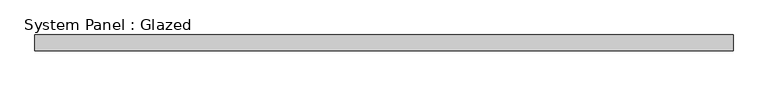
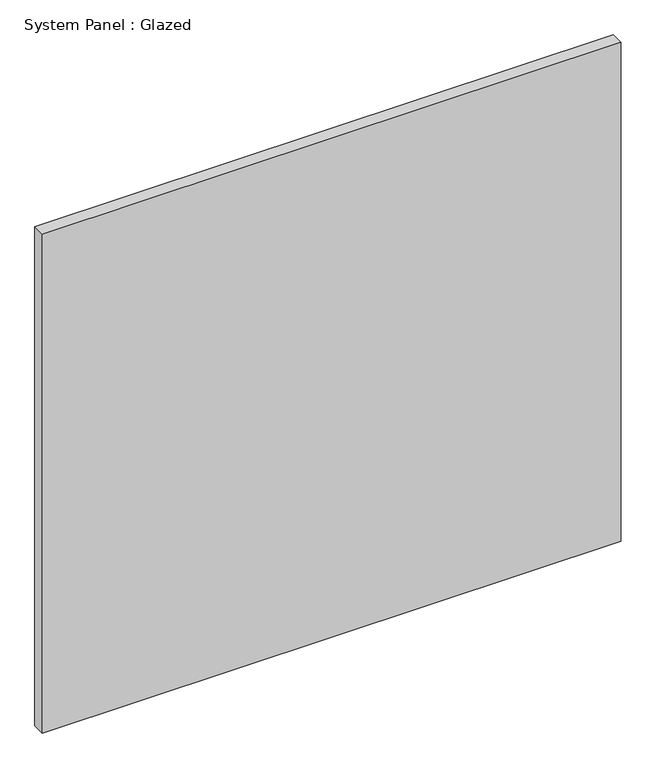
"""IFC4 building model written with IfcOpenShell, lengths in millimetres: plate geometry, System Panel : Glazed."""

from ifc_helpers import new_model, si_unit, origin, origin_with_axes, place, context, project, spatial, polyline, outline, extrude, source, transform, mapped, element, save


def system_panel_glazed_22820276(model_context):
    return source(origin(), model_context, "Body", "SweptSolid", [
        extrude(outline(polyline([(565.1500001, 19.05), (-565.1500001, 19.05), (-565.1500001, 44.45), (565.1500001, 44.45), (565.1500001, 19.05)])), origin_with_axes(), (0.0, 0.0, 1.0), 1030.2424454),
    ])


if __name__ == "__main__":
    model = new_model("IFC4")
    model_context = context("Model", 3, world=origin())
    ifc_project = project(units=[si_unit("LENGTHUNIT", "METRE", prefix="MILLI")], contexts=[model_context])
    site = spatial("IfcSite", under=ifc_project)
    building = spatial("IfcBuilding", under=site)
    placement = place(None, origin())
    system_panel_glazed_shape = system_panel_glazed_22820276(model_context)
    element("IfcPlate", 1, ObjectType="System Panel : Glazed", at=placement, inside=building, context=model_context, shape_type="MappedRepresentation", body=[
        mapped(system_panel_glazed_shape, transform((0.0, 0.0, 0.0), x_axis=(1.0, 0.0, 0.0), y_axis=(0.0, 1.0, 0.0), z_axis=(0.0, 0.0, 1.0))),
    ])
    save(model, "model.ifc")

# Revit data of these elements
# Type "System Panel : Glazed"
#   Construction Type Id = "GSP4R"
#   Analytic Construction = "1/8 in Pilkington single glazing"
#   Visual Light Transmittance = 0.9
#   Solar Heat Gain Coefficient = 0.86
#   Heat Transfer Coefficient (U) = 1.18115 BTU/(h·ft²·°F)
#   Define Thermal Properties by = 1
# Element 1 (IfcPlate, "System Panel : Glazed")
#   Materials on its faces: "Glass"
# Materials
#   "Glass": class "Glass", colour RGB 0 128 192, transparency 0.75, Description = "Soda Lime Glass", Cost = 0
